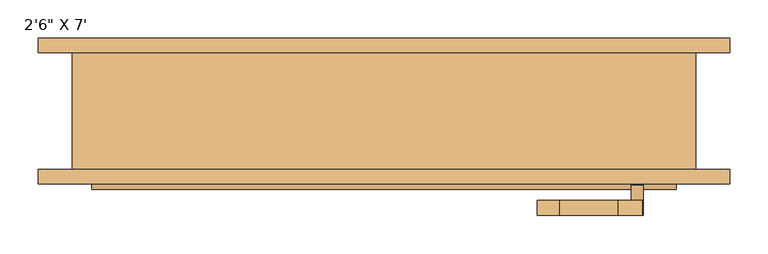
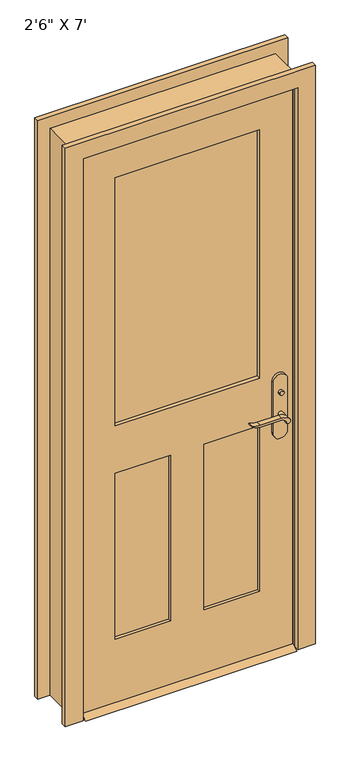
"""IFC4 building model written with IfcOpenShell, lengths in millimetres: door geometry."""

from ifc_helpers import new_model, si_unit, point, frame, frame_2d, origin, place, context, project, spatial, polyline, circle_curve, trimmed, segment, composite_curve, outline, extrude, faceted_brep, source, transform, mapped, element, save


def door_c9530512(model_context):
    return source(origin(), model_context, "Body", "SolidModel", [
        extrude(outline(polyline([(-38.1, 12.7), (-12.7, 0.0), (-98.425, 0.0), (-73.025, 12.7), (-38.1, 12.7)])), frame((-381.0, 0.0, 0.0), z_axis=(1.0, 0.0, 0.0), x_axis=(0.0, 1.0, 0.0)), (0.0, 0.0, 1.0), 762.0),
        extrude(outline(polyline([(335.2, -18.1), (335.2, -28.1), (325.2, -28.1), (325.2, -18.1), (335.2, -18.1)])), frame((0.0, 0.0, 981.9), z_axis=(0.0, 0.0, 1.0), x_axis=(1.0, 0.0, 0.0)), (0.0, 0.0, 1.0), 30.0),
        extrude(outline(composite_curve([segment(trimmed(circle_curve(frame_2d((996.9, 330.2)), 8.0), [point((996.9, 322.2))], [point((996.9, 338.2))], False, "CARTESIAN"), True, "CONTINUOUS"), segment(trimmed(circle_curve(frame_2d((996.9, 330.2)), 8.0), [point((996.9, 338.2))], [point((996.9, 322.2))], False, "CARTESIAN"), True, "CONTINUOUS")], self_intersect=False)), frame((0.0, -93.025, 0.0), z_axis=(0.0, 1.0, 0.0), x_axis=(0.0, 0.0, 1.0)), (0.0, 0.0, 1.0), 10.0),
        extrude(outline(composite_curve([segment(trimmed(circle_curve(frame_2d((897.1555521, 306.5324871)), 37.2832219), [point((919.0523287, 336.7081363))], [point((934.4, 304.8325667))], False, "CARTESIAN"), True, "CONTINUOUS"), segment(polyline([(934.4, 304.8325667), (934.4, 228.5564091)]), True, "CONTINUOUS"), segment(trimmed(circle_curve(frame_2d((1017.6850638, 228.6227909)), 83.2850902), [point((934.4, 228.5564091))], [point((939.4, 200.2))], True, "CARTESIAN"), True, "CONTINUOUS"), segment(polyline([(939.4, 200.2), (936.6135558, 200.2)]), True, "CONTINUOUS"), segment(trimmed(circle_curve(frame_2d((986.6709207, 232.1396612)), 59.3791355), [point((936.6135558, 200.2))], [point((927.4, 228.5564091))], False, "CARTESIAN"), True, "CONTINUOUS"), segment(polyline([(927.4, 228.5564091), (927.4, 304.8138099)]), True, "CONTINUOUS"), segment(trimmed(circle_curve(frame_2d((909.2738613, 304.8138099)), 18.1261387), [point((927.4, 304.8138099))], [point((914.4, 322.2))], True, "CARTESIAN"), True, "CONTINUOUS"), segment(trimmed(circle_curve(frame_2d((914.4, 330.2)), 8.0), [point((914.4, 322.2))], [point((919.0523287, 336.7081363))], False, "CARTESIAN"), True, "CONTINUOUS")], self_intersect=False)), frame((0.0, 1.9, 0.0), z_axis=(0.0, 1.0, 0.0), x_axis=(0.0, 0.0, 1.0)), (0.0, 0.0, 1.0), 20.0),
        extrude(outline(composite_curve([segment(trimmed(circle_curve(frame_2d((914.4, 330.2)), 8.0), [point((914.3999903, 322.2))], [point((919.0523287, 336.7081363))], False, "CARTESIAN"), True, "CONTINUOUS"), segment(trimmed(circle_curve(frame_2d((897.1555521, 306.5324871)), 37.2832219), [point((919.0523287, 336.7081363))], [point((934.4, 304.8325667))], False, "CARTESIAN"), True, "CONTINUOUS"), segment(polyline([(934.4, 304.8325667), (934.4, 228.5564091)]), True, "CONTINUOUS"), segment(trimmed(circle_curve(frame_2d((1017.6850638, 228.6227909)), 83.2850902), [point((934.4, 228.5564091))], [point((939.4, 200.2))], True, "CARTESIAN"), True, "CONTINUOUS"), segment(polyline([(939.4, 200.2), (936.6135558, 200.2)]), True, "CONTINUOUS"), segment(trimmed(circle_curve(frame_2d((986.6709207, 232.1396612)), 59.3791355), [point((936.6135558, 200.2))], [point((927.4, 228.5564091))], False, "CARTESIAN"), True, "CONTINUOUS"), segment(polyline([(927.4, 228.5564091), (927.4, 304.8138122)]), True, "CONTINUOUS"), segment(trimmed(circle_curve(frame_2d((909.2738682, 304.8138122)), 18.1261318), [point((927.4, 304.8138122))], [point((914.3999903, 322.2))], True, "CARTESIAN"), True, "CONTINUOUS")], self_intersect=False)), frame((0.0, -133.025, 0.0), z_axis=(0.0, 1.0, 0.0), x_axis=(0.0, 0.0, 1.0)), (0.0, 0.0, 1.0), 20.0),
        extrude(outline(composite_curve([segment(trimmed(circle_curve(frame_2d((914.4, 330.2)), 8.0), [point((914.4, 322.2))], [point((914.4, 338.2))], False, "CARTESIAN"), True, "CONTINUOUS"), segment(trimmed(circle_curve(frame_2d((914.4, 330.2)), 8.0), [point((914.4, 338.2))], [point((914.4, 322.2))], False, "CARTESIAN"), True, "CONTINUOUS")], self_intersect=False)), frame((0.0, -28.1, 0.0), z_axis=(0.0, 1.0, 0.0), x_axis=(0.0, 0.0, 1.0)), (0.0, 0.0, 1.0), 30.0),
        extrude(outline(composite_curve([segment(trimmed(circle_curve(frame_2d((914.4, 330.2)), 8.0), [point((914.4, 322.2))], [point((914.4, 338.2))], False, "CARTESIAN"), True, "CONTINUOUS"), segment(trimmed(circle_curve(frame_2d((914.4, 330.2)), 8.0), [point((914.4, 338.2))], [point((914.4, 322.2))], False, "CARTESIAN"), True, "CONTINUOUS")], self_intersect=False)), frame((0.0, -113.025, 0.0), z_axis=(0.0, 1.0, 0.0), x_axis=(0.0, 0.0, 1.0)), (0.0, 0.0, 1.0), 30.0),
        extrude(outline(composite_curve([segment(polyline([(844.4, 355.2), (1039.4, 355.2)]), True, "CONTINUOUS"), segment(trimmed(circle_curve(frame_2d((1039.4, 330.2)), 25.0), [point((1039.4, 355.2))], [point((1039.4, 305.2))], False, "CARTESIAN"), True, "CONTINUOUS"), segment(polyline([(1039.4, 305.2), (844.4, 305.2)]), True, "CONTINUOUS"), segment(trimmed(circle_curve(frame_2d((844.4, 330.2)), 25.0), [point((844.4, 305.2))], [point((844.4, 355.2))], False, "CARTESIAN"), True, "CONTINUOUS")], self_intersect=False)), frame((0.0, -38.1, 0.0), z_axis=(0.0, 1.0, 0.0), x_axis=(0.0, 0.0, 1.0)), (0.0, 0.0, 1.0), 10.0),
        extrude(outline(composite_curve([segment(polyline([(844.4, 355.2), (1039.4, 355.2)]), True, "CONTINUOUS"), segment(trimmed(circle_curve(frame_2d((1039.4, 330.2)), 25.0), [point((1039.4, 355.2))], [point((1039.4, 305.2))], False, "CARTESIAN"), True, "CONTINUOUS"), segment(polyline([(1039.4, 305.2), (844.4, 305.2)]), True, "CONTINUOUS"), segment(trimmed(circle_curve(frame_2d((844.4, 330.2)), 25.0), [point((844.4, 305.2))], [point((844.4, 355.2))], False, "CARTESIAN"), True, "CONTINUOUS")], self_intersect=False)), frame((0.0, -83.025, 0.0), z_axis=(0.0, 1.0, 0.0), x_axis=(0.0, 0.0, 1.0)), (0.0, 0.0, 1.0), 10.0),
        faceted_brep([(406.4, -73.025, 0.0), (381.0, -73.025, 0.0), (381.0, -38.1, 0.0), (368.3, -38.1, 0.0), (368.3, -3.175, 0.0), (381.0, -3.175, 0.0), (381.0, 79.375, 0.0), (406.4, 79.375, 0.0), (406.4, 79.375, 2159.0), (406.4, -73.025, 2159.0), (381.0, 79.375, 2133.6), (-381.0, 79.375, 2133.6), (-381.0, 79.375, 0.0), (-406.4, 79.375, 0.0), (-406.4, 79.375, 2159.0), (381.0, -3.175, 2133.6), (368.3, -3.175, 2120.9), (-368.3, -3.175, 2120.9), (-368.3, -3.175, 0.0), (-381.0, -3.175, 0.0), (-381.0, -3.175, 2133.6), (368.3, -38.1, 2120.9), (381.0, -38.1, 2133.6), (-381.0, -38.1, 2133.6), (-381.0, -38.1, 0.0), (-368.3, -38.1, 0.0), (-368.3, -38.1, 2120.9), (381.0, -73.025, 2133.6), (-406.4, -73.025, 2159.0), (-406.4, -73.025, 0.0), (-381.0, -73.025, 0.0), (-381.0, -73.025, 2133.6)], [[[0, 1, 2, 3, 4, 5, 6, 7]], [[7, 8, 9, 0]], [[6, 10, 11, 12, 13, 14, 8, 7]], [[5, 15, 10, 6]], [[4, 16, 17, 18, 19, 20, 15, 5]], [[3, 21, 16, 4]], [[2, 22, 23, 24, 25, 26, 21, 3]], [[1, 27, 22, 2]], [[0, 9, 28, 29, 30, 31, 27, 1]], [[8, 14, 28, 9]], [[15, 20, 11, 10]], [[21, 26, 17, 16]], [[27, 31, 23, 22]], [[29, 13, 12, 19, 18, 25, 24, 30]], [[14, 13, 29, 28]], [[20, 19, 12, 11]], [[26, 25, 18, 17]], [[31, 30, 24, 23]]]),
        extrude(outline(polyline([(2133.6, -381.0), (12.7, -381.0), (12.7, 381.0), (2133.6, 381.0), (2133.6, -381.0)]), holes=[polyline([(1066.8, -260.35), (2012.95, -260.35), (2012.95, 260.35), (1066.8, 260.35), (1066.8, -260.35)]), polyline([(885.825, -60.325), (254.0, -60.325), (254.0, -260.35), (885.825, -260.35), (885.825, -60.325)]), polyline([(885.825, 260.35), (254.0, 260.35), (254.0, 60.325), (885.825, 60.325), (885.825, 260.35)])]), frame((0.0, -73.025, 0.0), z_axis=(0.0, 1.0, 0.0), x_axis=(0.0, 0.0, 1.0)), (0.0, 0.0, 1.0), 34.925),
        extrude(outline(polyline([(260.35, -52.07), (260.35, -59.055), (-260.35, -59.055), (-260.35, -52.07), (260.35, -52.07)])), frame((0.0, 0.0, 1066.8), z_axis=(0.0, 0.0, 1.0), x_axis=(1.0, 0.0, 0.0)), (0.0, 0.0, 1.0), 946.15),
        extrude(outline(polyline([(-60.325, -49.7416667), (-60.325, -61.3833333), (-260.35, -61.3833333), (-260.35, -49.7416667), (-60.325, -49.7416667)])), frame((0.0, 0.0, 254.0), z_axis=(0.0, 0.0, 1.0), x_axis=(1.0, 0.0, 0.0)), (0.0, 0.0, 1.0), 631.825),
        extrude(outline(polyline([(260.35, -49.7416667), (260.35, -61.3833333), (60.325, -61.3833333), (60.325, -49.7416667), (260.35, -49.7416667)])), frame((0.0, 0.0, 254.0), z_axis=(0.0, 0.0, 1.0), x_axis=(1.0, 0.0, 0.0)), (0.0, 0.0, 1.0), 631.825),
        extrude(outline(polyline([(0.0, -387.35), (2139.95, -387.35), (2139.95, 387.35), (0.0, 387.35), (0.0, 450.85), (2203.45, 450.85), (2203.45, -450.85), (0.0, -450.85), (0.0, -387.35)])), frame((0.0, -92.075, 0.0), z_axis=(0.0, 1.0, 0.0), x_axis=(0.0, 0.0, 1.0)), (0.0, 0.0, 1.0), 19.05),
        extrude(outline(polyline([(0.0, -387.35), (2139.95, -387.35), (2139.95, 387.35), (0.0, 387.35), (0.0, 450.85), (2203.45, 450.85), (2203.45, -450.85), (0.0, -450.85), (0.0, -387.35)])), frame((0.0, 79.375, 0.0), z_axis=(0.0, 1.0, 0.0), x_axis=(0.0, 0.0, 1.0)), (0.0, 0.0, 1.0), 19.05),
    ])


if __name__ == "__main__":
    model = new_model("IFC4")
    model_context = context("Model", 3, world=origin())
    ifc_project = project(units=[si_unit("LENGTHUNIT", "METRE", prefix="MILLI")], contexts=[model_context])
    site = spatial("IfcSite", under=ifc_project)
    building = spatial("IfcBuilding", under=site)
    placement = place(None, origin())
    door_shape = door_c9530512(model_context)
    element("IfcDoor", 1, ObjectType="2'6\" X 7'", at=placement, inside=building, context=model_context, shape_type="MappedRepresentation", body=[
        mapped(door_shape, transform((0.0, 0.0, 0.0), x_axis=(1.0, 0.0, 0.0), y_axis=(0.0, 1.0, 0.0), z_axis=(0.0, 0.0, 1.0))),
    ])
    save(model, "model.ifc")

# Revit data of these elements
# Type "2'6\" X 7'"
#   Type Mark = "15"
#   Assembly Code = "B2030100"
#   Analytic Construction = "French door, wood frame with single glass"
#   Top Rail = 0' - 4 3/4"
#   Threshold Offset [instance default] = 0' - 0 1/2"
#   Thickness = 0' - 1 3/8"
#   Thermal Resistance (R) = 1.0696 (h·ft²·°F)/BTU
#   Swing Angle [instance default] = 90.00°
#   Stiles = 0' - 4 3/4"
#   Rough Width = 2' - 8"
#   Rough Height = 7' - 1"
#   Lock Rail = 0' - 7 1/8"
#   Height = 7' - 0"
#   Width = 2' - 6"
#   Heat Transfer Coefficient (U) = 0.9350 BTU/(h·ft²·°F)
#   Door Offset [instance default] = 0' - 0"
#   Bottom Rail = 0' - 9 1/2"
#   Threshold [instance default] = yes
#   Function = 1
#   Exterior Trim [instance default] = yes
#   Trim Material = Cherry
#   Threshold Material = Cherry
#   Panel Material = Cherry
#   Glazing = Glass
#   Frame Material = Cherry
#   Door Handle Material = Aluminum
#   Visual Light Transmittance = 0
#   Solar Heat Gain Coefficient = 0
#   Wall Closure = (empty or 0)
#   Construction Type = (empty or 0)
# Element 1 (IfcDoor, "2'6\" X 7'")
#   Materials on its faces: "Cherry", "Aluminum", "Glass"
# Materials
#   "Cherry": class "Wood", colour RGB 226 177 128, transparency 0, Description = "Prunus Serotina", Cost = 0
#   "Glass": class "Glass", colour RGB 0 128 192, transparency 0.75, Description = "Soda Lime Glass", Cost = 0
#   "Aluminum": class "Metal", colour RGB 247 247 247, transparency 0, Description = "Aluminum 6061", Cost = 0
